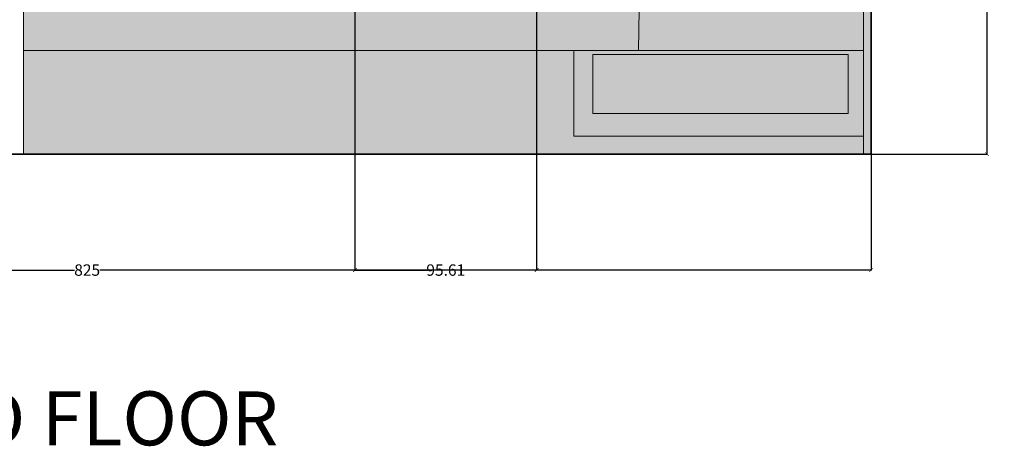
# Model space of a CAD drawing. Units: inches. Extents: x 1704 to 6393, y -157 to 1172.
# Tile 23 of 122: x 2275 to 2793, y -157 to 67. Entities that reach past the tile are written whole.
import ezdxf

# ---------------------------------------------------------------- set-up
doc = ezdxf.new("R2010")
doc.units = ezdxf.units.IN
doc.header["$MEASUREMENT"] = 0
for name, color, linetype, lineweight in [('A-ANNO-DIMS', 7, 'Continuous', 13), ('A-ANNO-TEXT', 7, 'Continuous', 25), ('A-WALL-PATT', 7, 'Continuous', 13), ('C-PROP', 7, 'Continuous', 35), ('L-HRDS', 8, 'Continuous', 18), ('L-PVMT-PATT', 8, 'Continuous', 13)]:
    doc.layers.add(name, color=color, linetype=linetype, lineweight=lineweight)
doc.layers.add('L-HRDS-PATT', color=9, linetype='Continuous', lineweight=13, true_color=0xc5c1ba)
doc.layers.add('L-PLNT-PATT', color=253, linetype='Continuous', lineweight=13, true_color=0x9abc8f)
doc.styles.get("Standard").update_dxf_attribs({"font": 'arial.ttf'})
doc.dimstyles.get("Standard").update_dxf_attribs({"dimtxt": 6, "dimasz": 2, "dimexe": 0.18, "dimexo": 0.0625, "dimgap": 0.09, "dimtad": 0, "dimtih": 1, "dimtoh": 1, "dimdec": 1, "dimzin": 0, "dimdsep": 46, "dimlunit": 3, "dimtxsty": 'Standard', "dimblk": 'ARCHTICK', "dimcen": 0.09, "dimadec": 0, "dimazin": 0, "dimtfac": 1, "dimtdec": 1, "dimtofl": 0, "dimtmove": 0, "dimatfit": 3, "dimfxl": 1, "dimtolj": 1, "dimtzin": 0, "dimarcsym": 0})

# ---------------------------------------------------------------- blocks, each defined once
blk = doc.blocks.new('_ArchTick')
at = {"color": 0, "linetype": 'ByBlock', "const_width": 0.15}
blk.add_lwpolyline([(-0.5, -0.5), (0.5, 0.5)], dxfattribs=at)
blk = doc.blocks.new('*D90')
at = {"layer": 'A-ANNO-DIMS', "color": 0, "lineweight": -2, "transparency": 16777216}
for p, q in [((1898.35, -3.85), (1898.35, -64.97)), ((2723.35, -3.85), (2723.35, -64.97)), ((1898.35, -64.79), (2304.1, -64.79)), ((2723.35, -64.79), (2317.59, -64.79))]:
    blk.add_line(p, q, dxfattribs=at)
at = {"layer": 'Defpoints', "color": 0, "lineweight": -3, "transparency": 16777216}
for p in [(1898.35, -3.79), (2723.35, -3.79), (2723.35, -64.79)]:
    blk.add_point(p, dxfattribs=at)
at = {"layer": 'A-ANNO-DIMS', "color": 0, "lineweight": -2, "transparency": 16777216, "xscale": 2, "yscale": 2, "zscale": 2, "rotation": 180}
blk.add_blockref('_ArchTick', (1898.35, -64.79), dxfattribs=at)
at = {"layer": 'A-ANNO-DIMS', "color": 0, "lineweight": -2, "transparency": 16777216, "xscale": 2, "yscale": 2, "zscale": 2}
blk.add_blockref('_ArchTick', (2723.35, -64.79), dxfattribs=at)
at = {"layer": 'A-ANNO-DIMS', "color": 0, "transparency": 16777216, "insert": (2310.85, -64.79), "char_height": 6, "attachment_point": 5}
blk.add_mtext('\\A1;825', dxfattribs=at)
blk = doc.blocks.new('*D91')
at = {"layer": 'A-ANNO-DIMS', "color": 0, "lineweight": -2, "transparency": 16777216}
for p, q in [((2723.41, 1033.21), (2784.53, 1033.21)), ((2784.35, 1033.21), (2784.35, 517.87)), ((2784.35, -3.79), (2784.35, 511.56)), ((2723.41, -3.79), (2784.53, -3.79))]:
    blk.add_line(p, q, dxfattribs=at)
at = {"layer": 'Defpoints', "color": 0, "lineweight": -3, "transparency": 16777216}
for p in [(2723.35, 1033.21), (2784.35, 1033.21), (2723.35, -3.79)]:
    blk.add_point(p, dxfattribs=at)
at = {"layer": 'A-ANNO-DIMS', "color": 0, "lineweight": -2, "transparency": 16777216, "xscale": 2, "yscale": 2, "zscale": 2}
for p, rotation in [((2784.35, 1033.21), 90), ((2784.35, -3.79), 270)]:
    blk.add_blockref('_ArchTick', p, dxfattribs=dict(at, rotation=rotation))
at = {"layer": 'A-ANNO-DIMS', "color": 0, "transparency": 16777216, "insert": (2784.35, 514.71), "char_height": 6, "attachment_point": 5}
blk.add_mtext('\\A1;1037', dxfattribs=at)
blk = doc.blocks.new('*D105')
at = {"layer": 'A-ANNO-DIMS', "color": 0, "lineweight": -2, "transparency": 16777216}
for p, q in [((2451.74, 615.15), (2451.74, -64.97)), ((2547.35, 615.15), (2547.35, -64.97)), ((2451.74, -64.79), (2489.91, -64.79)), ((2547.35, -64.79), (2509.18, -64.79))]:
    blk.add_line(p, q, dxfattribs=at)
at = {"layer": 'Defpoints', "color": 0, "lineweight": -3, "transparency": 16777216}
for p in [(2451.74, 615.21), (2547.35, 615.21), (2547.35, -64.79)]:
    blk.add_point(p, dxfattribs=at)
at = {"layer": 'A-ANNO-DIMS', "color": 0, "lineweight": -2, "transparency": 16777216, "xscale": 2, "yscale": 2, "zscale": 2, "rotation": 180}
blk.add_blockref('_ArchTick', (2451.74, -64.79), dxfattribs=at)
at = {"layer": 'A-ANNO-DIMS', "color": 0, "lineweight": -2, "transparency": 16777216, "xscale": 2, "yscale": 2, "zscale": 2}
blk.add_blockref('_ArchTick', (2547.35, -64.79), dxfattribs=at)
at = {"layer": 'A-ANNO-DIMS', "color": 0, "transparency": 16777216, "insert": (2499.54, -64.79), "char_height": 6, "attachment_point": 5}
blk.add_mtext('\\A1;95.61', dxfattribs=at)

msp = doc.modelspace()

# ---------------------------------------------------------------- hatches: boundary and pattern name
at = {"layer": 'A-WALL-PATT', "transparency": 33554643}
h = msp.add_hatch(color=256, dxfattribs=at)
h.dxf.hatch_style = 1
h.paths.add_polyline_path([(2723.349, 368.213), (2719.349, 368.213), (2719.349, 5.658), (2719.349, -3.787), (2723.349, -3.787)])
at = {"layer": 'L-HRDS-PATT', "transparency": 33554539}
h = msp.add_hatch(color=256, dxfattribs=at)
h.dxf.hatch_style = 1
h.paths.add_polyline_path([(2651.217, 368.213), (2605.349, 368.213), (2605.349, 218.213), (2605.349, 212.464), (2605.349, 210.513), (2605.349, 153.913), (2605.349, 151.962), (2605.349, 146.213), (2605.349, 90.213), (2605.349, 72.213), (2601.349, 72.213), (2600.88, 50.634), (2719.349, 50.634), (2719.349, 72.213), (2711.349, 72.213), (2663.217, 72.213), (2651.217, 72.213)])
h.paths.add_polyline_path([(2711.349, 48.634), (2600.88, 48.634), (2576.88, 48.634), (2576.88, 17.658), (2711.349, 17.658)])
h.paths.add_polyline_path([(2601.349, 72.213), (2597.349, 72.213), (2597.349, 90.213), (2429.349, 90.213), (2425.516, 90.213), (2424.215, 90.213), (2386.482, 90.213), (2385.181, 90.213), (2381.349, 90.213), (2357.349, 90.213), (2357.349, 72.213), (2349.349, 72.213), (2349.349, 90.213), (2349.349, 134.213), (2277.349, 134.213), (2277.349, 50.634), (2566.88, 50.634), (2600.88, 50.634)])
h.paths.add_polyline_path([(2349.349, 146.213), (2277.349, 146.213), (2277.349, 134.213), (2349.349, 134.213)])
h.paths.add_polyline_path([(2349.349, 158.213), (2277.349, 158.213), (2277.349, 146.213), (2349.349, 146.213)])
h.paths.add_polyline_path([(2349.349, 170.213), (2277.349, 170.213), (2277.349, 158.213), (2349.349, 158.213)])
h.paths.add_polyline_path([(2349.349, 194.213), (2337.349, 194.213), (2337.349, 202.213), (2349.349, 202.213), (2349.349, 364.213), (2277.349, 364.213), (2277.349, 202.213), (2289.349, 202.213), (2289.349, 194.213), (2277.349, 194.213), (2277.349, 170.213), (2349.349, 170.213)])
at = {"layer": 'L-PLNT-PATT', "transparency": 33554643}
h = msp.add_hatch(color=256, dxfattribs=at)
h.dxf.hatch_style = 1
h.paths.add_polyline_path([(2566.88, 50.634), (2277.349, 50.634), (2277.349, -3.787), (2719.349, -3.787), (2719.349, 5.658), (2566.88, 5.658)])
at = {"layer": 'L-PVMT-PATT', "transparency": 33554643}
h = msp.add_hatch(dxfattribs=at)
h.set_pattern_fill('GRAVEL', color=256, scale=2.4)
h.set_pattern_definition([(228.0127875, (1.728, 2.4), (-19.2, -21.6), [0.3228864, -31.9658113]), (184.9697407, (1.512, 2.16), (28.8, 2.4), [0.5540832, -54.8542194]), (132.510447, (0.96, 2.112), (24, -26.4), [0.3906912, -38.6784782]), (267.273689, (0.024, 1.512), (2.4, 48), [0.5045712, -49.9525393]), (292.833654, (0, 1.008), (-12, 28.8), [0.494772, -48.9824955]), (357.273689, (0.192, 0.552), (-48, 2.4), [0.5045712, -49.9525393]), (37.6942405, (0.696, 0.528), (-31.2, -24), [0.6672696, -66.0596365]), (72.2553284, (1.224, 0.936), (16.8, 52.8), [0.6299712, -62.3671716]), (121.4295656, (1.416, 1.536), (-19.2, 31.2), [0.50628, -50.1217755]), (175.236358, (1.152, 1.968), (26.4, -2.4), [0.5779968, -28.3218302]), (222.3974378, (0.576, 2.016), (-28.8, -26.4), [0.7474752, -74.0001]), (138.814075, (2.4, 1.488), (-16.8, 14.4), [0.2551224, -25.2572276]), (171.4692344, (2.208, 1.656), (31.2, -4.8), [0.4853688, -48.0516274]), (225, (1.728, 1.728), (-3e-16, -2.4), [0.3394104, -3.0547021]), (203.19859, (1.56, 2.016), (12, 4.8), [0.1827792, -18.0950763]), (291.80141, (1.392, 1.944), (-2.4, 7.2), [0.2584872, -12.6659083]), (30.963757, (1.488, 1.704), (7.2, 4.8), [0.4198296, -13.574455]), (161.56505, (1.848, 1.92), (4.8, -2.4), [0.3035784, -7.285888]), (16.3895403, (0, 1.944), (24, 7.2), [0.42528, -42.1028284]), (70.346176, (0.408, 2.064), (-9.6, -26.4), [0.3567864, -35.3217786]), (293.19859, (1.848, 2.4), (-4.8, 12), [0.365556, -17.9122995]), (343.6104597, (1.992, 2.064), (-24, 7.2), [0.42528, -42.1028284]), (339.443955, (0, 0.456), (-12, 4.8), [0.410112, -20.095497]), (294.7751406, (0.384, 0.312), (-12, 26.4), [0.3436272, -34.0191434]), (66.80141, (1.872, 0), (4.8, 12), [0.365556, -17.9122995]), (17.3540246, (2.016, 0.336), (-31.2, -9.6), [0.4023144, -39.8290167]), (69.443955, (0.696, 0), (-4.8, -12), [0.205056, -20.300553]), (101.309932, (1.728, 0), (-2.4, 9.6), [0.122376, -12.1152708]), (165.963757, (1.704, 0.12), (7.2, -2.4), [0.494772, -9.4006815]), (186.009006, (1.224, 0.24), (24, 2.4), [0.45852, -45.3934156]), (303.690068, (1.488, 1.488), (-2.4, 4.8), [0.3461328, -8.3071903]), (353.1572266, (1.68, 1.2), (40.8, -4.8), [0.6043056, -59.8261503]), (60.945396, (2.28, 1.128), (-9.6, -16.8), [0.2470944, -24.462418]), (90, (2.4, 1.344), (-2.4, 2.4), [0.144, -2.256]), (120.256437, (1.176, 0.312), (9.6, -16.8), [0.3334176, -33.008448]), (48.0127875, (1.008, 0.6), (19.2, 21.6), [0.6457728, -31.642925]), (0, (1.44, 1.08), (2.4, 2.4), [0.624, -1.776]), (325.3048465, (2.064, 1.08), (24, -16.8), [0.3794736, -37.5678583]), (254.054604, (2.376, 0.864), (-2.4, -9.6), [0.3494448, -17.122819]), (207.6459754, (2.28, 0.528), (-45.6, -24), [0.568956, -56.326738]), (175.4260787, (1.776, 0.264), (-31.2, 2.4), [0.6019176, -59.5897762])])
h.paths.add_polyline_path([(2719.349, 368.213), (2711.349, 368.213), (2711.349, 318.481), (2663.217, 318.481), (2663.217, 368.213), (2651.217, 368.213), (2651.217, 72.213), (2663.217, 72.213), (2663.217, 137.213), (2711.349, 137.213), (2711.349, 72.213), (2663.217, 72.213), (2651.217, 72.213), (2651.217, 368.213), (2605.349, 368.213), (2605.349, 218.213), (2605.349, 212.464), (2605.349, 210.513), (2605.349, 153.913), (2605.349, 151.962), (2605.349, 146.213), (2605.349, 90.213), (2605.349, 72.213), (2601.349, 72.213), (2600.88, 50.634), (2277.349, 50.634), (2277.349, -3.787), (2719.349, -3.787)])
h.paths.add_polyline_path([(2663.217, 272.481), (2711.349, 272.481), (2711.349, 207.213), (2663.217, 207.213)], flags=16)
h.paths.add_polyline_path([(2663.217, 202.213), (2711.349, 202.213), (2711.349, 142.213), (2663.217, 142.213)], flags=16)
h.paths.add_polyline_path([(2663.217, 277.481), (2663.217, 313.481), (2711.349, 313.481), (2711.349, 277.481)], flags=16)
h = msp.add_hatch(dxfattribs=at)
h.set_pattern_fill('GRAVEL', color=256, scale=6)
h.set_pattern_definition([(228.012788, (4.32, 6), (-48, -54), [0.807216, -79.914528]), (184.969741, (3.78, 5.4), (72, 6), [1.385208, -137.135549]), (132.510447, (2.4, 5.28), (60, -66), [0.976728, -96.696196]), (267.273689, (0.06, 3.78), (6, 120), [1.261428, -124.881348]), (292.833654, (0, 2.52), (-30, 72), [1.23693, -122.456239]), (357.273689, (0.48, 1.38), (-120, 6), [1.261428, -124.881348]), (37.6942405, (1.74, 1.32), (-78, -60), [1.668174, -165.149091]), (72.255328, (3.06, 2.34), (42, 132), [1.574928, -155.917929]), (121.429566, (3.54, 3.84), (-48, 78), [1.2657, -125.304439]), (175.236358, (2.88, 4.92), (66, -6), [1.444992, -70.804575]), (222.397438, (1.44, 5.04), (-72, -66), [1.868688, -185.00025]), (138.814075, (6, 3.72), (-42, 36), [0.637806, -63.143069]), (171.469234, (5.52, 4.14), (78, -12), [1.213422, -120.129068]), (225, (4.32, 4.32), (-7e-16, -6), [0.848526, -7.636755]), (203.19859, (3.9, 5.04), (30, 12), [0.456948, -45.23769]), (291.80141, (3.48, 4.86), (-6, 18), [0.646218, -31.664771]), (30.963757, (3.72, 4.26), (18, 12), [1.049574, -33.936137]), (161.56505, (4.62, 4.8), (12, -6), [0.758946, -18.21472]), (16.38954, (0, 4.86), (60, 18), [1.0632, -105.257071]), (70.346176, (1.02, 5.16), (-24, -66), [0.891966, -88.304446]), (293.19859, (4.62, 6), (-12, 30), [0.91389, -44.780749]), (343.61046, (4.98, 5.16), (-60, 18), [1.0632, -105.257071]), (339.443955, (0, 1.14), (-30, 12), [1.02528, -50.238742]), (294.77514, (0.96, 0.78), (-30, 66), [0.859068, -85.047858]), (66.80141, (4.68, 0), (12, 30), [0.91389, -44.780749]), (17.354025, (5.04, 0.84), (-78, -24), [1.005786, -99.572542]), (69.443955, (1.74, 0), (-12, -30), [0.51264, -50.751382]), (101.30993, (4.32, 0), (-6, 24), [0.30594, -30.288177]), (165.963757, (4.26, 0.3), (18, -6), [1.23693, -23.501704]), (186.009006, (3.06, 0.6), (60, 6), [1.1463, -113.483539]), (303.69007, (3.72, 3.72), (-6, 12), [0.865332, -20.767976]), (353.157227, (4.2, 3), (102, -12), [1.510764, -149.565376]), (60.945396, (5.7, 2.82), (-24, -42), [0.617736, -61.156045]), (90, (6, 3.36), (-6, 6), [0.36, -5.64]), (120.256437, (2.94, 0.78), (24, -42), [0.833544, -82.52112]), (48.012788, (2.52, 1.5), (48, 54), [1.614432, -79.107312]), (0, (3.6, 2.7), (6, 6), [1.56, -4.44]), (325.304846, (5.16, 2.7), (60, -42), [0.948684, -93.919646]), (254.054604, (5.94, 2.16), (-6, -24), [0.873612, -42.807047]), (207.645975, (5.7, 1.32), (-114, -60), [1.42239, -140.816845]), (175.426079, (4.44, 0.66), (-78, 6), [1.504794, -148.97444])])
h.paths.add_polyline_path([(2719.349, 50.634), (2600.88, 50.634), (2566.88, 50.634), (2566.88, 5.658), (2719.349, 5.658)])
h.paths.add_polyline_path([(2576.88, 48.634), (2600.88, 48.634), (2711.349, 48.634), (2711.349, 17.658), (2576.88, 17.658)], flags=16)

# ---------------------------------------------------------------- linework, layer by layer
at = {"layer": 'C-PROP'}
for q in [(2723.349, 1033.213), (1898.349, -3.787)]:
    msp.add_line((2723.349, -3.787), q, dxfattribs=at)
at = {"layer": 'L-HRDS'}
for p, q in [((2719.349, 5.658), (2719.349, 1033.213)), ((2277.349, 194.213), (2277.349, -3.787)), ((2601.349, 72.213), (2600.88, 50.634)), ((2566.88, 50.634), (2277.349, 50.634)), ((2600.88, 50.634), (2566.88, 50.634)), ((2566.88, 50.634), (2566.88, 5.658)), ((2600.88, 48.634), (2576.88, 48.634)), ((2576.88, 48.634), (2576.88, 17.658)), ((2600.88, 50.634), (2719.349, 50.634)), ((2600.88, 48.634), (2711.349, 48.634)), ((2711.349, 17.658), (2711.349, 48.634)), ((2576.88, 17.658), (2711.349, 17.658)), ((2566.88, 5.658), (2719.349, 5.658)), ((2719.349, 5.658), (2719.349, -3.787))]:
    msp.add_line(p, q, dxfattribs=at)

# ---------------------------------------------------------------- texts
at = {"layer": 'A-ANNO-TEXT'}
msp.add_text('GROUND FLOOR', height=28.38733, dxfattribs=at).set_placement((2115.73, -156.99))

# ---------------------------------------------------------------- dimensions: what is measured, and where the dimension line sits
at = {"layer": 'A-ANNO-DIMS'}
dim = msp.add_linear_dim(base=(2784.349, 1033.213), p1=(2723.349, -3.787), p2=(2723.349, 1033.213), angle=90, dimstyle='Standard', override={"dimdec": 0, "dimlfac": 1, "dimrnd": 0, "dimzin": 0, "dimdsep": 46, "dimlunit": 2}, dxfattribs=at)
dim.commit()
dim.dimension.update_dxf_attribs({"geometry": '*D91', "text_midpoint": (2784.349, 514.713)})
for base, p1, p2, override, picture, middle in [((2547.349, -64.787), (2451.738, 615.213), (2547.349, 615.213), {"dimdec": 2, "dimlfac": 1, "dimrnd": 0, "dimzin": 0, "dimdsep": 46, "dimlunit": 2}, '*D105', (2499.543, -64.787)), ((2723.349, -64.787), (1898.349, -3.787), (2723.349, -3.787), {"dimdec": 0, "dimlfac": 1, "dimrnd": 0, "dimzin": 0, "dimdsep": 46, "dimlunit": 2}, '*D90', (2310.849, -64.787))]:
    dim = msp.add_linear_dim(base=base, p1=p1, p2=p2, dimstyle='Standard', override=override, dxfattribs=at)
    dim.commit()
    dim.dimension.update_dxf_attribs({"geometry": picture, "text_midpoint": middle})

doc.saveas('drawing.dxf')
